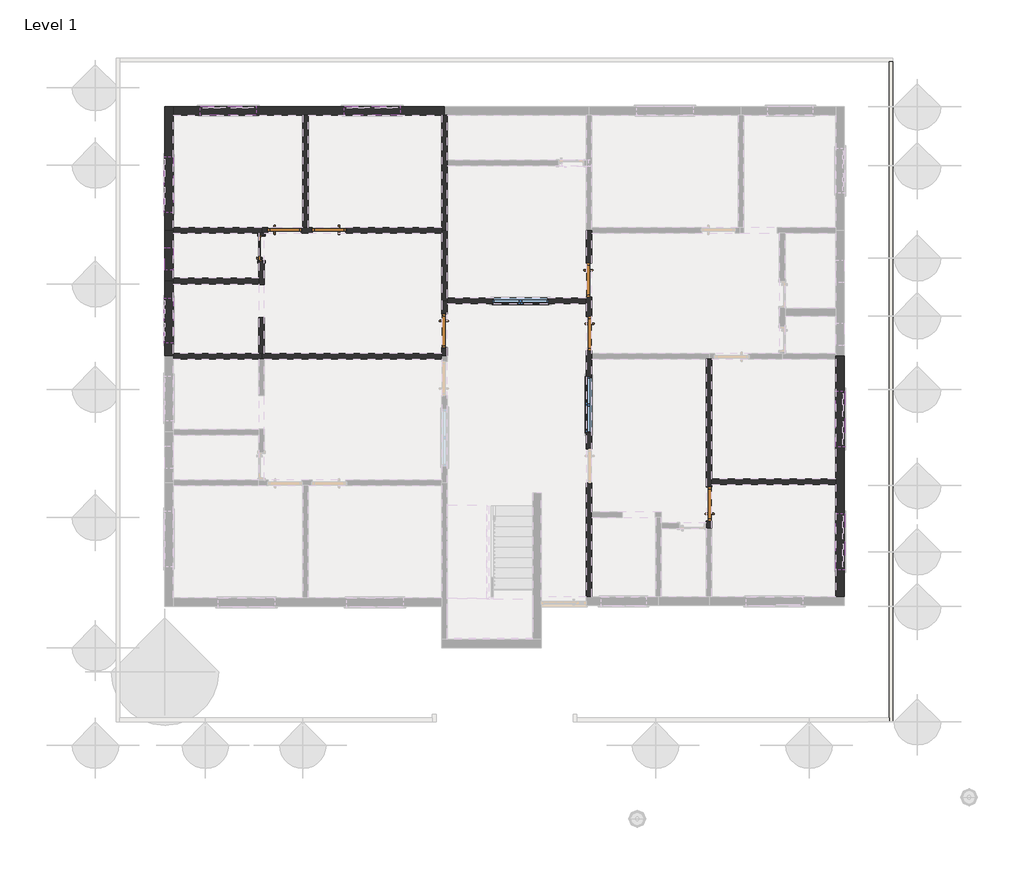
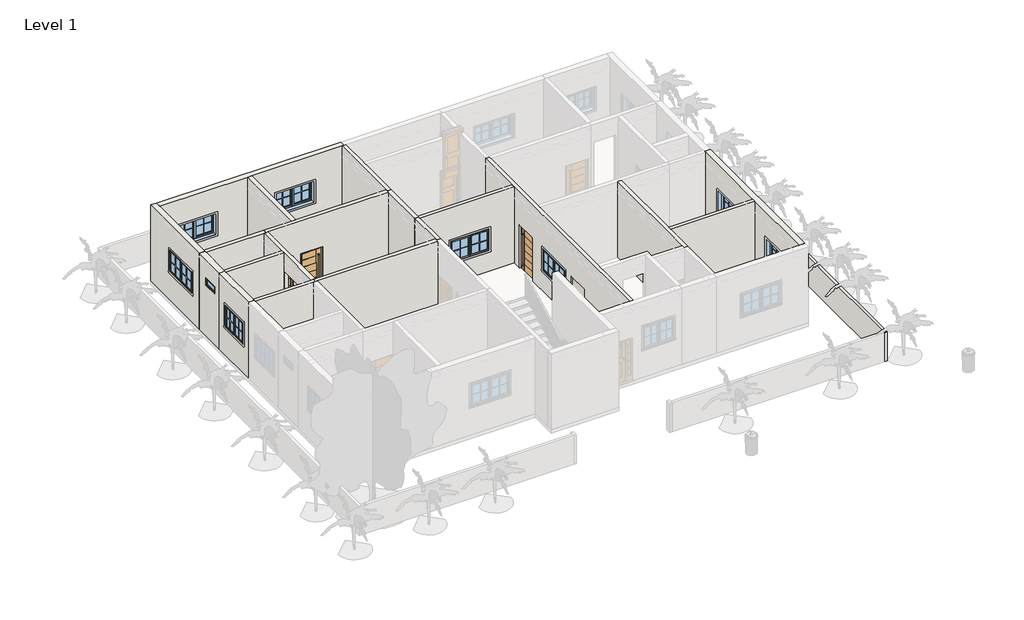
# One storey, part 2 of 5: 20 walls, 9 windows, 7 doors.
"""IFC4 building model written with IfcOpenShell, lengths in millimetres."""

from ifc_helpers import new_model, si_unit, origin, origin_with_axes, place, context, project, spatial, polyline, outline, extrude, faceted_brep, transform, mapped, element, save
from components import door_3_ad1505b7, door_3_44036f4b, door_57d9c04c, fixed_2_d9cafb20, m_window_awning_double_horizontal_4_0c6a2509, m_window_awning_double_horizontal_5_7c720334, m_window_awning_double_horizontal_5_337400f2

model = new_model("IFC4")

# Units and contexts
model_context = context("Model", 3, world=origin())
ifc_project = project(units=[si_unit("LENGTHUNIT", "METRE", prefix="MILLI")], contexts=[model_context])

# Site, building, storey
site = spatial("IfcSite", under=ifc_project)
building = spatial("IfcBuilding", under=site)
storey = spatial("IfcBuildingStorey", under=building, Name="Level 1", Elevation=0.0)

# Doors
placement = place(None, origin())
door_3_shape = door_3_ad1505b7(model_context)
element("IfcDoor", 1, ObjectType="3'", at=placement, inside=storey, context=model_context, shape_type="MappedRepresentation", body=[
    mapped(door_3_shape, transform((-21766.1847893, 19978.1922903, 0.0), x_axis=(1.0, 0.0, 0.0), y_axis=(0.0, 1.0, 0.0), z_axis=(0.0, 0.0, 1.0))),
])
element("IfcDoor", 2, ObjectType="3'", at=placement, inside=storey, context=model_context, shape_type="MappedRepresentation", body=[
    mapped(door_3_shape, transform((-13523.8847893, 17184.1922903, 0.0), x_axis=(0.0, -1.0, 0.0), y_axis=(1.0, 0.0, 0.0), z_axis=(0.0, 0.0, 1.0))),
])
door_3_2_shape = door_3_44036f4b(model_context)
element("IfcDoor", 3, ObjectType="3'", at=placement, inside=storey, context=model_context, shape_type="MappedRepresentation", body=[
    mapped(door_3_2_shape, transform((-20559.6847893, 19978.1922903, 0.0), x_axis=(-1.0, 0.0, 0.0), y_axis=(0.0, -1.0, 0.0), z_axis=(0.0, 0.0, 1.0))),
])
element("IfcDoor", 4, ObjectType="3'", at=placement, inside=storey, context=model_context, shape_type="MappedRepresentation", body=[
    mapped(door_3_2_shape, transform((-17435.4847893, 17260.3922903, 0.0), x_axis=(0.0, -1.0, 0.0), y_axis=(1.0, 0.0, 0.0), z_axis=(0.0, 0.0, 1.0))),
])
element("IfcDoor", 5, ObjectType="3'", at=placement, inside=storey, context=model_context, shape_type="MappedRepresentation", body=[
    mapped(door_3_2_shape, transform((-13523.8847893, 18631.9922903, 0.0), x_axis=(0.0, -1.0, 0.0), y_axis=(1.0, 0.0, 0.0), z_axis=(0.0, 0.0, 1.0))),
])
element("IfcDoor", 6, ObjectType="3'", at=placement, inside=storey, context=model_context, shape_type="MappedRepresentation", body=[
    mapped(door_3_2_shape, transform((-10272.6847893, 12574.0922903, 0.0), x_axis=(0.0, 1.0, 0.0), y_axis=(-1.0, 0.0, 0.0), z_axis=(0.0, 0.0, 1.0))),
])
door_shape = door_57d9c04c(model_context)
element("IfcDoor", 7, ObjectType="M_Door-Interior-Single-2_Panel-Wood : 2'2\"", at=placement, inside=storey, context=model_context, shape_type="MappedRepresentation", body=[
    mapped(door_shape, transform((-22391.6597893, 19495.5922903, 0.0), x_axis=(0.0, 1.0, 0.0), y_axis=(-1.0, 0.0, 0.0), z_axis=(0.0, 0.0, 1.0))),
])

# Walls
element("IfcWall", 8, ObjectType="Generic - 4\"", at=placement, inside=storey, context=model_context, shape_type="Brep", body=[
    faceted_brep([(-5395.8847893, 24550.1922903, -152.4), (-5395.8847893, 6770.1922903, -152.4), (-5395.8847893, 6668.5922903, -152.4), (-5395.8847893, 6668.5922903, 1066.8), (-5395.8847893, 6770.1922903, 1066.8), (-5395.8847893, 24550.1922903, 1066.8), (-5294.2847893, 24550.1922903, -152.4), (-5294.2847893, 24550.1922903, 1066.8), (-5294.2847893, 6668.5922903, 1066.8), (-5294.2847893, 6668.5922903, -152.4)], [[[0, 1, 2, 3, 4, 5]], [[6, 7, 8, 9]], [[2, 1, 0, 6, 9]], [[5, 4, 3, 8, 7]], [[0, 5, 7, 6]], [[3, 2, 9, 8]]]),
])
element("IfcWall", 9, ObjectType="Generic - 6\"", at=placement, inside=storey, context=model_context, shape_type="Brep", body=[
    faceted_brep([(-17511.6847893, 23102.3922903, 0.0), (-17511.6847893, 20054.3922903, 0.0), (-17511.6847893, 19978.1922903, 0.0), (-17511.6847893, 19978.1922903, 3200.4), (-17511.6847893, 20054.3922903, 3200.4), (-17511.6847893, 23102.3922903, 3200.4), (-17359.2847893, 23102.3922903, 0.0), (-17359.2847893, 23102.3922903, 3200.4), (-17359.2847893, 21883.1922903, 3200.4), (-17359.2847893, 21730.7922903, 3200.4), (-17359.2847893, 19978.1922903, 3200.4), (-17359.2847893, 19978.1922903, 0.0), (-17359.2847893, 21730.7922903, 0.0), (-17359.2847893, 21883.1922903, 0.0), (-17435.4847893, 23102.3922903, 0.0), (-17435.4847893, 23102.3922903, 3200.4)], [[[0, 1, 2, 3, 4, 5]], [[6, 7, 8, 9, 10, 11, 12, 13]], [[2, 1, 0, 14, 6, 13, 12, 11]], [[3, 2, 11, 10]], [[5, 4, 3, 10, 9, 8, 7, 15]], [[0, 5, 15, 7, 6, 14]]]),
])
element("IfcWall", 10, ObjectType="Generic - 6\"", at=placement, inside=storey, context=model_context, shape_type="Brep", body=[
    faceted_brep([(-24776.0847893, 19901.9922903, 0.0), (-22464.6847893, 19901.9922903, 0.0), (-22388.4847893, 19901.9922903, 0.0), (-22388.4847893, 19901.9922903, 3200.4), (-22464.6847893, 19901.9922903, 3200.4), (-24776.0847893, 19901.9922903, 3200.4), (-24776.0847893, 20054.3922903, 0.0), (-24776.0847893, 20054.3922903, 3200.4), (-22388.4847893, 20054.3922903, 3200.4), (-22388.4847893, 20054.3922903, 0.0), (-24776.0847893, 19978.1922903, 0.0), (-24776.0847893, 19978.1922903, 3200.4)], [[[0, 1, 2, 3, 4, 5]], [[6, 7, 8, 9]], [[2, 1, 0, 10, 6, 9]], [[3, 2, 9, 8]], [[5, 4, 3, 8, 7, 11]], [[0, 5, 11, 7, 6, 10]]]),
])
element("IfcWall", 11, ObjectType="Generic - 6\"", at=placement, inside=storey, context=model_context, shape_type="SweptSolid", body=[
    extrude(outline(polyline([(-21270.8847893, 20054.3922903), (-21270.8847893, 23102.3922903), (-21118.4847893, 23102.3922903), (-21118.4847893, 20054.3922903), (-21270.8847893, 20054.3922903)])), origin_with_axes(), (0.0, 0.0, 1.0), 3200.4),
])
element("IfcWall", 12, ObjectType="Generic - 6\"", at=placement, inside=storey, context=model_context, shape_type="Brep", body=[
    faceted_brep([(-24776.0847893, 16498.3922903, 0.0), (-22464.6847893, 16498.3922903, 0.0), (-22388.4847893, 16498.3922903, 0.0), (-22388.4847893, 16498.3922903, 3200.4), (-22464.6847893, 16498.3922903, 3200.4), (-24776.0847893, 16498.3922903, 3200.4), (-24776.0847893, 16650.7922903, 0.0), (-24776.0847893, 16650.7922903, 3200.4), (-22464.6847893, 16650.7922903, 3200.4), (-22388.4847893, 16650.7922903, 3200.4), (-22388.4847893, 16650.7922903, 0.0), (-22464.6847893, 16650.7922903, 0.0), (-24776.0847893, 16574.5922903, 0.0), (-24776.0847893, 16574.5922903, 3200.4)], [[[0, 1, 2, 3, 4, 5]], [[6, 7, 8, 9, 10, 11]], [[2, 1, 0, 12, 6, 11, 10]], [[3, 2, 10, 9]], [[5, 4, 3, 9, 8, 7, 13]], [[0, 5, 13, 7, 6, 12]]]),
])
element("IfcWall", 13, ObjectType="Generic - 6\"", at=placement, inside=storey, context=model_context, shape_type="Brep", body=[
    faceted_brep([(-24776.0847893, 18530.3922903, 0.0), (-22464.6847893, 18530.3922903, 0.0), (-22464.6847893, 18530.3922903, 3200.4), (-24776.0847893, 18530.3922903, 3200.4), (-24776.0847893, 18682.7922903, 0.0), (-24776.0847893, 18682.7922903, 3200.4), (-22464.6847893, 18682.7922903, 3200.4), (-22464.6847893, 18682.7922903, 0.0), (-24776.0847893, 18606.5922903, 0.0), (-24776.0847893, 18606.5922903, 3200.4)], [[[0, 1, 2, 3]], [[4, 5, 6, 7]], [[1, 0, 8, 4, 7]], [[3, 2, 6, 5, 9]], [[0, 3, 9, 5, 4, 8]], [[2, 1, 7, 6]]]),
])
element("IfcWall", 14, ObjectType="Generic - 6\"", at=placement, inside=storey, context=model_context, shape_type="Brep", body=[
    faceted_brep([(-22312.2847893, 19901.9922903, 3200.4), (-22312.2847893, 16650.7922903, 3200.4), (-22312.2847893, 16650.7922903, 0.0), (-22312.2847893, 17622.2018411, 0.0), (-22312.2847893, 17622.2018411, 2438.4), (-22312.2847893, 18518.7795946, 2438.4), (-22312.2847893, 18518.7795946, 0.0), (-22312.2847893, 19140.3922903, 0.0), (-22312.2847893, 19140.3922903, 1853.8), (-22312.2847893, 19850.7922903, 1853.8), (-22312.2847893, 19850.7922903, 0.0), (-22312.2847893, 19901.9922903, 0.0), (-22464.6847893, 16650.7922903, 3200.4), (-22464.6847893, 18530.3922903, 3200.4), (-22464.6847893, 18682.7922903, 3200.4), (-22464.6847893, 19901.9922903, 3200.4), (-22464.6847893, 19901.9922903, 0.0), (-22464.6847893, 19850.7922903, 0.0), (-22464.6847893, 19850.7922903, 1853.8), (-22464.6847893, 19140.3922903, 1853.8), (-22464.6847893, 19140.3922903, 0.0), (-22464.6847893, 18682.7922903, 0.0), (-22464.6847893, 18530.3922903, 0.0), (-22464.6847893, 18518.7795946, 0.0), (-22464.6847893, 18518.7795946, 2438.4), (-22464.6847893, 17622.2018411, 2438.4), (-22464.6847893, 17622.2018411, 0.0), (-22464.6847893, 16650.7922903, 0.0), (-22388.4847893, 16650.7922903, 0.0), (-22388.4847893, 19901.9922903, 0.0), (-22388.4847893, 19901.9922903, 3200.4), (-22388.4847893, 16650.7922903, 3200.4)], [[[0, 1, 2, 3, 4, 5, 6, 7, 8, 9, 10, 11]], [[12, 13, 14, 15, 16, 17, 18, 19, 20, 21, 22, 23, 24, 25, 26, 27]], [[2, 28, 27, 26, 3]], [[6, 23, 22, 21, 20, 7]], [[16, 29, 11, 10, 17]], [[1, 0, 30, 15, 14, 13, 12, 31]], [[0, 11, 29, 16, 15, 30]], [[2, 1, 31, 12, 27, 28]], [[9, 18, 17, 10]], [[18, 9, 8, 19]], [[19, 8, 7, 20]], [[4, 25, 24, 5]], [[25, 4, 3, 26]], [[5, 24, 23, 6]]]),
])
element("IfcWall", 15, ObjectType="Generic - 6\"", at=placement, inside=storey, context=model_context, shape_type="Brep", body=[
    faceted_brep([(-17359.2847893, 17996.9922903, 0.0), (-13600.0847893, 17996.9922903, 0.0), (-13600.0847893, 17996.9922903, 3200.4), (-17359.2847893, 17996.9922903, 3200.4), (-16140.0847893, 17996.9922903, 1814.4), (-14616.0847893, 17996.9922903, 1814.4), (-14616.0847893, 17996.9922903, 900.0), (-16140.0847893, 17996.9922903, 900.0), (-17359.2847893, 18149.3922903, 0.0), (-17359.2847893, 18149.3922903, 3200.4), (-13600.0847893, 18149.3922903, 3200.4), (-13600.0847893, 18149.3922903, 0.0), (-16140.0847893, 18149.3922903, 1814.4), (-16140.0847893, 18149.3922903, 900.0), (-14616.0847893, 18149.3922903, 900.0), (-14616.0847893, 18149.3922903, 1814.4), (-17359.2847893, 18073.1922903, 0.0), (-17359.2847893, 18073.1922903, 3200.4)], [[[0, 1, 2, 3], [4, 5, 6, 7]], [[8, 9, 10, 11], [12, 13, 14, 15]], [[1, 0, 16, 8, 11]], [[3, 2, 10, 9, 17]], [[0, 3, 17, 9, 8, 16]], [[2, 1, 11, 10]], [[13, 12, 4, 7]], [[14, 13, 7, 6]], [[15, 14, 6, 5]], [[12, 15, 5, 4]]]),
])
element("IfcWall", 16, ObjectType="Generic - 6\"", at=placement, inside=storey, context=model_context, shape_type="Brep", body=[
    faceted_brep([(-10348.8847893, 11913.6922903, 0.0), (-10348.8847893, 11913.6922903, 3200.4), (-10348.8847893, 12053.3922903, 3200.4), (-10348.8847893, 16498.3922903, 3200.4), (-10348.8847893, 16498.3922903, 0.0), (-10348.8847893, 13031.2922903, 0.0), (-10348.8847893, 13031.2922903, 1828.8), (-10348.8847893, 12116.8922903, 1828.8), (-10348.8847893, 12116.8922903, 0.0), (-10348.8847893, 12053.3922903, 0.0), (-10196.4847893, 11913.6922903, 3200.4), (-10196.4847893, 11913.6922903, 0.0), (-10196.4847893, 12116.8922903, 0.0), (-10196.4847893, 12116.8922903, 1828.8), (-10196.4847893, 13031.2922903, 1828.8), (-10196.4847893, 13031.2922903, 0.0), (-10196.4847893, 13094.7922903, 0.0), (-10196.4847893, 13247.1922903, 0.0), (-10196.4847893, 16498.3922903, 0.0), (-10196.4847893, 16498.3922903, 3200.4), (-10196.4847893, 13247.1922903, 3200.4), (-10196.4847893, 13094.7922903, 3200.4), (-10272.6847893, 16498.3922903, 0.0), (-10216.4847893, 13031.2922903, 0.0), (-10216.4847893, 13046.2922903, 0.0), (-10293.4847893, 13046.2922903, 0.0), (-10293.4847893, 13031.2922903, 0.0), (-10293.4847893, 12116.8922903, 0.0), (-10293.4847893, 12101.8922903, 0.0), (-10216.4847893, 12101.8922903, 0.0), (-10216.4847893, 12116.8922903, 0.0), (-10272.6847893, 16498.3922903, 3200.4), (-10216.4847893, 12116.8922903, 1828.8), (-10216.4847893, 13031.2922903, 1828.8), (-10293.4847893, 13031.2922903, 1828.8), (-10293.4847893, 12116.8922903, 1828.8), (-10216.4847893, 12101.8922903, 1843.8), (-10293.4847893, 12101.8922903, 1843.8), (-10293.4847893, 13046.2922903, 1843.8), (-10216.4847893, 13046.2922903, 1843.8)], [[[0, 1, 2, 3, 4, 5, 6, 7, 8, 9]], [[10, 11, 12, 13, 14, 15, 16, 17, 18, 19, 20, 21]], [[4, 22, 18, 17, 16, 15, 23, 24, 25, 26, 5]], [[11, 0, 9, 8, 27, 28, 29, 30, 12]], [[1, 0, 11, 10]], [[3, 2, 1, 10, 21, 20, 19, 31]], [[4, 3, 31, 19, 18, 22]], [[13, 32, 33, 14]], [[6, 34, 35, 7]], [[14, 33, 23, 15]], [[34, 6, 5, 26]], [[32, 13, 12, 30]], [[7, 35, 27, 8]], [[36, 37, 38, 39]], [[39, 38, 25, 24]], [[35, 34, 26, 25, 38, 37, 28, 27]], [[37, 36, 29, 28]], [[33, 32, 30, 29, 36, 39, 24, 23]]]),
])
element("IfcWall", 17, ObjectType="Generic - 6\"", at=placement, inside=storey, context=model_context, shape_type="SweptSolid", body=[
    extrude(outline(polyline([(-6843.6847893, 13094.7922903), (-10196.4847893, 13094.7922903), (-10196.4847893, 13247.1922903), (-6843.6847893, 13247.1922903), (-6843.6847893, 13094.7922903)])), origin_with_axes(), (0.0, 0.0, 1.0), 3200.4),
])
element("IfcWall", 18, ObjectType="Generic - 6\"", at=placement, inside=storey, context=model_context, shape_type="Brep", body=[
    faceted_brep([(-13600.0847893, 10046.7922903, 3200.4), (-13600.0847893, 17996.9922903, 3200.4), (-13600.0847893, 18149.3922903, 3200.4), (-13600.0847893, 19978.1922903, 3200.4), (-13600.0847893, 19978.1922903, 0.0), (-13600.0847893, 19089.1922903, 0.0), (-13600.0847893, 19089.1922903, 1828.8), (-13600.0847893, 18174.7922903, 1828.8), (-13600.0847893, 18174.7922903, 0.0), (-13600.0847893, 18149.3922903, 0.0), (-13600.0847893, 17996.9922903, 0.0), (-13600.0847893, 17641.3922903, 0.0), (-13600.0847893, 17641.3922903, 1828.8), (-13600.0847893, 16726.9922903, 1828.8), (-13600.0847893, 16726.9922903, 0.0), (-13600.0847893, 14059.9922903, 0.0), (-13600.0847893, 14059.9922903, 1828.8), (-13600.0847893, 13145.5922903, 1828.8), (-13600.0847893, 13145.5922903, 0.0), (-13600.0847893, 10046.7922903, 0.0), (-13600.0847893, 10046.7922903, 1828.8), (-13600.0847893, 16015.7922903, 1814.4), (-13600.0847893, 14491.7922903, 1814.4), (-13600.0847893, 14491.7922903, 900.0), (-13600.0847893, 16015.7922903, 900.0), (-13447.6847893, 19978.1922903, 3200.4), (-13447.6847893, 19901.9922903, 3200.4), (-13447.6847893, 16650.7922903, 3200.4), (-13447.6847893, 16498.3922903, 3200.4), (-13447.6847893, 12358.1922903, 3200.4), (-13447.6847893, 12205.7922903, 3200.4), (-13447.6847893, 10046.7922903, 3200.4), (-13447.6847893, 10046.7922903, 0.0), (-13447.6847893, 12205.7922903, 0.0), (-13447.6847893, 12358.1922903, 0.0), (-13447.6847893, 13145.5922903, 0.0), (-13447.6847893, 13145.5922903, 1828.8), (-13447.6847893, 14059.9922903, 1828.8), (-13447.6847893, 14059.9922903, 0.0), (-13447.6847893, 16498.3922903, 0.0), (-13447.6847893, 16650.7922903, 0.0), (-13447.6847893, 16726.9922903, 0.0), (-13447.6847893, 16726.9922903, 1828.8), (-13447.6847893, 17641.3922903, 1828.8), (-13447.6847893, 17641.3922903, 0.0), (-13447.6847893, 18174.7922903, 0.0), (-13447.6847893, 18174.7922903, 1828.8), (-13447.6847893, 19089.1922903, 1828.8), (-13447.6847893, 19089.1922903, 0.0), (-13447.6847893, 19901.9922903, 0.0), (-13447.6847893, 19978.1922903, 0.0), (-13447.6847893, 16015.7922903, 1814.4), (-13447.6847893, 16015.7922903, 900.0), (-13447.6847893, 14491.7922903, 900.0), (-13447.6847893, 14491.7922903, 1814.4), (-13544.6847893, 13145.5922903, 0.0), (-13544.6847893, 13130.5922903, 0.0), (-13467.6847893, 13130.5922903, 0.0), (-13467.6847893, 13145.5922903, 0.0), (-13544.6847893, 14059.9922903, 0.0), (-13544.6847893, 16726.9922903, 0.0), (-13544.6847893, 16711.9922903, 0.0), (-13467.6847893, 16711.9922903, 0.0), (-13467.6847893, 16726.9922903, 0.0), (-13467.6847893, 14059.9922903, 0.0), (-13467.6847893, 14074.9922903, 0.0), (-13544.6847893, 14074.9922903, 0.0), (-13544.6847893, 17641.3922903, 0.0), (-13580.0847893, 18174.7922903, 0.0), (-13580.0847893, 18159.7922903, 0.0), (-13503.0847893, 18159.7922903, 0.0), (-13503.0847893, 18174.7922903, 0.0), (-13467.6847893, 17641.3922903, 0.0), (-13467.6847893, 17656.3922903, 0.0), (-13544.6847893, 17656.3922903, 0.0), (-13503.0847893, 19089.1922903, 0.0), (-13503.0847893, 19104.1922903, 0.0), (-13580.0847893, 19104.1922903, 0.0), (-13580.0847893, 19089.1922903, 0.0), (-13544.6847893, 14059.9922903, 1828.8), (-13544.6847893, 13145.5922903, 1828.8), (-13467.6847893, 14059.9922903, 1828.8), (-13467.6847893, 13145.5922903, 1828.8), (-13467.6847893, 14074.9922903, 1843.8), (-13467.6847893, 13130.5922903, 1843.8), (-13544.6847893, 13130.5922903, 1843.8), (-13544.6847893, 14074.9922903, 1843.8), (-13544.6847893, 17641.3922903, 1828.8), (-13544.6847893, 16726.9922903, 1828.8), (-13467.6847893, 17641.3922903, 1828.8), (-13467.6847893, 16726.9922903, 1828.8), (-13467.6847893, 17656.3922903, 1843.8), (-13467.6847893, 16711.9922903, 1843.8), (-13544.6847893, 16711.9922903, 1843.8), (-13544.6847893, 17656.3922903, 1843.8), (-13580.0847893, 19089.1922903, 1828.8), (-13580.0847893, 18174.7922903, 1828.8), (-13503.0847893, 18174.7922903, 1828.8), (-13503.0847893, 19089.1922903, 1828.8), (-13580.0847893, 19104.1922903, 1843.8), (-13503.0847893, 19104.1922903, 1843.8), (-13503.0847893, 18159.7922903, 1843.8), (-13580.0847893, 18159.7922903, 1843.8)], [[[0, 1, 2, 3, 4, 5, 6, 7, 8, 9, 10, 11, 12, 13, 14, 15, 16, 17, 18, 19, 20], [21, 22, 23, 24]], [[25, 26, 27, 28, 29, 30, 31, 32, 33, 34, 35, 36, 37, 38, 39, 40, 41, 42, 43, 44, 45, 46, 47, 48, 49, 50], [51, 52, 53, 54]], [[32, 19, 18, 55, 56, 57, 58, 35, 34, 33]], [[59, 15, 14, 60, 61, 62, 63, 41, 40, 39, 38, 64, 65, 66]], [[67, 11, 10, 9, 8, 68, 69, 70, 71, 45, 44, 72, 73, 74]], [[4, 50, 49, 48, 75, 76, 77, 78, 5]], [[3, 2, 1, 0, 31, 30, 29, 28, 27, 26, 25]], [[4, 3, 25, 50]], [[0, 20, 19, 32, 31]], [[16, 79, 80, 17]], [[81, 37, 36, 82]], [[17, 80, 55, 18]], [[82, 36, 35, 58]], [[79, 16, 15, 59]], [[37, 81, 64, 38]], [[83, 84, 85, 86]], [[85, 84, 57, 56]], [[86, 85, 56, 55, 80, 79, 59, 66]], [[83, 86, 66, 65]], [[84, 83, 65, 64, 81, 82, 58, 57]], [[12, 87, 88, 13]], [[89, 43, 42, 90]], [[13, 88, 60, 14]], [[90, 42, 41, 63]], [[87, 12, 11, 67]], [[43, 89, 72, 44]], [[91, 92, 93, 94]], [[93, 92, 62, 61]], [[94, 93, 61, 60, 88, 87, 67, 74]], [[91, 94, 74, 73]], [[92, 91, 73, 72, 89, 90, 63, 62]], [[6, 95, 96, 7]], [[46, 97, 98, 47]], [[97, 46, 45, 71]], [[7, 96, 68, 8]], [[47, 98, 75, 48]], [[95, 6, 5, 78]], [[99, 100, 101, 102]], [[102, 101, 70, 69]], [[98, 97, 71, 70, 101, 100, 76, 75]], [[100, 99, 77, 76]], [[96, 95, 78, 77, 99, 102, 69, 68]], [[51, 54, 22, 21]], [[54, 53, 23, 22]], [[53, 52, 24, 23]], [[52, 51, 21, 24]]]),
])
element("IfcWall", 19, ObjectType="Generic - 6\"", at=placement, inside=storey, context=model_context, shape_type="Brep", body=[
    faceted_brep([(-22388.4847893, 16498.3922903, 0.0), (-22312.2847893, 16498.3922903, 0.0), (-17511.6847893, 16498.3922903, 0.0), (-17511.6847893, 16498.3922903, 3200.4), (-22312.2847893, 16498.3922903, 3200.4), (-22388.4847893, 16498.3922903, 3200.4), (-22388.4847893, 16650.7922903, 0.0), (-22388.4847893, 16650.7922903, 3200.4), (-22312.2847893, 16650.7922903, 3200.4), (-17511.6847893, 16650.7922903, 3200.4), (-17511.6847893, 16650.7922903, 0.0), (-22312.2847893, 16650.7922903, 0.0), (-17511.6847893, 16574.5922903, 0.0), (-17511.6847893, 16574.5922903, 3200.4)], [[[0, 1, 2, 3, 4, 5]], [[6, 7, 8, 9, 10, 11]], [[2, 1, 0, 6, 11, 10, 12]], [[5, 4, 3, 13, 9, 8, 7]], [[0, 5, 7, 6]], [[3, 2, 12, 10, 9, 13]]]),
])
element("IfcWall", 20, ObjectType="Generic - 6\"", at=placement, inside=storey, context=model_context, shape_type="Brep", body=[
    faceted_brep([(-17511.6847893, 19978.1922903, 0.0), (-17511.6847893, 19901.9922903, 0.0), (-17511.6847893, 18073.1922903, 0.0), (-17511.6847893, 18073.1922903, 3200.4), (-17511.6847893, 19901.9922903, 3200.4), (-17511.6847893, 19978.1922903, 3200.4), (-17359.2847893, 19978.1922903, 0.0), (-17359.2847893, 19978.1922903, 3200.4), (-17359.2847893, 18149.3922903, 3200.4), (-17359.2847893, 18073.1922903, 3200.4), (-17359.2847893, 18073.1922903, 0.0), (-17359.2847893, 18149.3922903, 0.0)], [[[0, 1, 2, 3, 4, 5]], [[6, 7, 8, 9, 10, 11]], [[2, 1, 0, 6, 11, 10]], [[3, 2, 10, 9]], [[5, 4, 3, 9, 8, 7]], [[0, 5, 7, 6]]]),
])
element("IfcWall", 21, ObjectType="Generic - 6\"", at=placement, inside=storey, context=model_context, shape_type="Brep", body=[
    faceted_brep([(-17511.6847893, 19901.9922903, 3200.4), (-22312.2847893, 19901.9922903, 3200.4), (-22388.4847893, 19901.9922903, 3200.4), (-22388.4847893, 19901.9922903, 0.0), (-22312.2847893, 19901.9922903, 0.0), (-22223.3847893, 19901.9922903, 0.0), (-22223.3847893, 19901.9922903, 1828.8), (-21308.9847893, 19901.9922903, 1828.8), (-21308.9847893, 19901.9922903, 0.0), (-21016.8847893, 19901.9922903, 0.0), (-21016.8847893, 19901.9922903, 1828.8), (-20102.4847893, 19901.9922903, 1828.8), (-20102.4847893, 19901.9922903, 0.0), (-17511.6847893, 19901.9922903, 0.0), (-22388.4847893, 20054.3922903, 3200.4), (-21270.8847893, 20054.3922903, 3200.4), (-21118.4847893, 20054.3922903, 3200.4), (-17511.6847893, 20054.3922903, 3200.4), (-17511.6847893, 20054.3922903, 0.0), (-20102.4847893, 20054.3922903, 0.0), (-20102.4847893, 20054.3922903, 1828.8), (-21016.8847893, 20054.3922903, 1828.8), (-21016.8847893, 20054.3922903, 0.0), (-21118.4847893, 20054.3922903, 0.0), (-21270.8847893, 20054.3922903, 0.0), (-21308.9847893, 20054.3922903, 0.0), (-21308.9847893, 20054.3922903, 1828.8), (-22223.3847893, 20054.3922903, 1828.8), (-22223.3847893, 20054.3922903, 0.0), (-22388.4847893, 20054.3922903, 0.0), (-17511.6847893, 19978.1922903, 0.0), (-20102.4847893, 19957.3922903, 0.0), (-20087.4847893, 19957.3922903, 0.0), (-20087.4847893, 20034.3922903, 0.0), (-20102.4847893, 20034.3922903, 0.0), (-21308.9847893, 19957.3922903, 0.0), (-21293.9847893, 19957.3922903, 0.0), (-21293.9847893, 20034.3922903, 0.0), (-21308.9847893, 20034.3922903, 0.0), (-21016.8847893, 20034.3922903, 0.0), (-21031.8847893, 20034.3922903, 0.0), (-21031.8847893, 19957.3922903, 0.0), (-21016.8847893, 19957.3922903, 0.0), (-22223.3847893, 20034.3922903, 0.0), (-22238.3847893, 20034.3922903, 0.0), (-22238.3847893, 19957.3922903, 0.0), (-22223.3847893, 19957.3922903, 0.0), (-17511.6847893, 19978.1922903, 3200.4), (-22223.3847893, 19957.3922903, 1828.8), (-21308.9847893, 19957.3922903, 1828.8), (-22223.3847893, 20034.3922903, 1828.8), (-21308.9847893, 20034.3922903, 1828.8), (-22238.3847893, 20034.3922903, 1843.8), (-21293.9847893, 20034.3922903, 1843.8), (-21293.9847893, 19957.3922903, 1843.8), (-22238.3847893, 19957.3922903, 1843.8), (-20102.4847893, 20034.3922903, 1828.8), (-21016.8847893, 20034.3922903, 1828.8), (-21016.8847893, 19957.3922903, 1828.8), (-20102.4847893, 19957.3922903, 1828.8), (-20087.4847893, 20034.3922903, 1843.8), (-20087.4847893, 19957.3922903, 1843.8), (-21031.8847893, 19957.3922903, 1843.8), (-21031.8847893, 20034.3922903, 1843.8)], [[[0, 1, 2, 3, 4, 5, 6, 7, 8, 9, 10, 11, 12, 13]], [[14, 15, 16, 17, 18, 19, 20, 21, 22, 23, 24, 25, 26, 27, 28, 29]], [[18, 30, 13, 12, 31, 32, 33, 34, 19]], [[8, 35, 36, 37, 38, 25, 24, 23, 22, 39, 40, 41, 42, 9]], [[3, 29, 28, 43, 44, 45, 46, 5, 4]], [[2, 1, 0, 47, 17, 16, 15, 14]], [[3, 2, 14, 29]], [[0, 13, 30, 18, 17, 47]], [[6, 48, 49, 7]], [[50, 27, 26, 51]], [[7, 49, 35, 8]], [[51, 26, 25, 38]], [[48, 6, 5, 46]], [[27, 50, 43, 28]], [[52, 53, 54, 55]], [[54, 53, 37, 36]], [[55, 54, 36, 35, 49, 48, 46, 45]], [[52, 55, 45, 44]], [[53, 52, 44, 43, 50, 51, 38, 37]], [[20, 56, 57, 21]], [[10, 58, 59, 11]], [[58, 10, 9, 42]], [[21, 57, 39, 22]], [[11, 59, 31, 12]], [[56, 20, 19, 34]], [[60, 61, 62, 63]], [[63, 62, 41, 40]], [[59, 58, 42, 41, 62, 61, 32, 31]], [[61, 60, 33, 32]], [[57, 56, 34, 33, 60, 63, 40, 39]]]),
])
element("IfcWall", 22, ObjectType="Generic - 6\"", at=placement, inside=storey, context=model_context, shape_type="Brep", body=[
    faceted_brep([(-17511.6847893, 16574.5922903, 0.0), (-17511.6847893, 16574.5922903, 3200.4), (-17511.6847893, 16650.7922903, 3200.4), (-17511.6847893, 18073.1922903, 3200.4), (-17511.6847893, 18073.1922903, 0.0), (-17511.6847893, 17717.5922903, 0.0), (-17511.6847893, 17717.5922903, 1828.8), (-17511.6847893, 16803.1922903, 1828.8), (-17511.6847893, 16803.1922903, 0.0), (-17511.6847893, 16650.7922903, 0.0), (-17359.2847893, 16574.5922903, 3200.4), (-17359.2847893, 16574.5922903, 0.0), (-17359.2847893, 16803.1922903, 0.0), (-17359.2847893, 16803.1922903, 1828.8), (-17359.2847893, 17717.5922903, 1828.8), (-17359.2847893, 17717.5922903, 0.0), (-17359.2847893, 17996.9922903, 0.0), (-17359.2847893, 18073.1922903, 0.0), (-17359.2847893, 18073.1922903, 3200.4), (-17359.2847893, 17996.9922903, 3200.4), (-17414.6847893, 17717.5922903, 0.0), (-17414.6847893, 17732.5922903, 0.0), (-17491.6847893, 17732.5922903, 0.0), (-17491.6847893, 17717.5922903, 0.0), (-17491.6847893, 16803.1922903, 0.0), (-17491.6847893, 16788.1922903, 0.0), (-17414.6847893, 16788.1922903, 0.0), (-17414.6847893, 16803.1922903, 0.0), (-17491.6847893, 17717.5922903, 1828.8), (-17491.6847893, 16803.1922903, 1828.8), (-17414.6847893, 16803.1922903, 1828.8), (-17414.6847893, 17717.5922903, 1828.8), (-17491.6847893, 17732.5922903, 1843.8), (-17414.6847893, 17732.5922903, 1843.8), (-17414.6847893, 16788.1922903, 1843.8), (-17491.6847893, 16788.1922903, 1843.8)], [[[0, 1, 2, 3, 4, 5, 6, 7, 8, 9]], [[10, 11, 12, 13, 14, 15, 16, 17, 18, 19]], [[4, 17, 16, 15, 20, 21, 22, 23, 5]], [[11, 0, 9, 8, 24, 25, 26, 27, 12]], [[1, 0, 11, 10]], [[3, 2, 1, 10, 19, 18]], [[4, 3, 18, 17]], [[6, 28, 29, 7]], [[13, 30, 31, 14]], [[30, 13, 12, 27]], [[7, 29, 24, 8]], [[14, 31, 20, 15]], [[28, 6, 5, 23]], [[32, 33, 34, 35]], [[35, 34, 26, 25]], [[31, 30, 27, 26, 34, 33, 21, 20]], [[33, 32, 22, 21]], [[29, 28, 23, 22, 32, 35, 25, 24]]]),
])
element("IfcWall", 23, ObjectType="Generic - 9\"", at=placement, inside=storey, context=model_context, shape_type="Brep", body=[
    faceted_brep([(-25004.6847893, 23330.9922903, 0.0), (-25004.6847893, 19978.1922903, 0.0), (-25004.6847893, 19978.1922903, 3200.4), (-25004.6847893, 23330.9922903, 3200.4), (-25004.6847893, 21984.7922903, 2133.5570313), (-25004.6847893, 20460.7922903, 2133.5570313), (-25004.6847893, 20460.7922903, 1219.1570313), (-25004.6847893, 21984.7922903, 1219.1570313), (-24776.0847893, 23330.9922903, 0.0), (-24776.0847893, 23330.9922903, 3200.4), (-24776.0847893, 23102.3922903, 3200.4), (-24776.0847893, 20054.3922903, 3200.4), (-24776.0847893, 19978.1922903, 3200.4), (-24776.0847893, 19978.1922903, 0.0), (-24776.0847893, 20054.3922903, 0.0), (-24776.0847893, 23102.3922903, 0.0), (-24776.0847893, 21984.7922903, 2133.5570313), (-24776.0847893, 21984.7922903, 1219.1570313), (-24776.0847893, 20460.7922903, 1219.1570313), (-24776.0847893, 20460.7922903, 2133.5570313)], [[[0, 1, 2, 3], [4, 5, 6, 7]], [[8, 9, 10, 11, 12, 13, 14, 15], [16, 17, 18, 19]], [[1, 0, 8, 15, 14, 13]], [[2, 1, 13, 12]], [[3, 2, 12, 11, 10, 9]], [[0, 3, 9, 8]], [[17, 16, 4, 7]], [[18, 17, 7, 6]], [[19, 18, 6, 5]], [[16, 19, 5, 4]]]),
])
element("IfcWall", 24, ObjectType="Generic - 9\"", at=placement, inside=storey, context=model_context, shape_type="Brep", body=[
    faceted_brep([(-6615.0847893, 10046.7922903, 0.0), (-6615.0847893, 16574.5922903, 0.0), (-6615.0847893, 16574.5922903, 3200.4), (-6615.0847893, 10046.7922903, 3200.4), (-6615.0847893, 10789.7422903, 2133.5570313), (-6615.0847893, 12313.7422903, 2133.5570313), (-6615.0847893, 12313.7422903, 1219.1570313), (-6615.0847893, 10789.7422903, 1219.1570313), (-6615.0847893, 14110.7922903, 2133.5570313), (-6615.0847893, 15634.7922903, 2133.5570313), (-6615.0847893, 15634.7922903, 1219.1570313), (-6615.0847893, 14110.7922903, 1219.1570313), (-6843.6847893, 10046.7922903, 0.0), (-6843.6847893, 10046.7922903, 3200.4), (-6843.6847893, 13094.7922903, 3200.4), (-6843.6847893, 13247.1922903, 3200.4), (-6843.6847893, 16498.3922903, 3200.4), (-6843.6847893, 16574.5922903, 3200.4), (-6843.6847893, 16574.5922903, 0.0), (-6843.6847893, 16498.3922903, 0.0), (-6843.6847893, 13247.1922903, 0.0), (-6843.6847893, 13094.7922903, 0.0), (-6843.6847893, 10789.7422903, 2133.5570313), (-6843.6847893, 10789.7422903, 1219.1570313), (-6843.6847893, 12313.7422903, 1219.1570313), (-6843.6847893, 12313.7422903, 2133.5570313), (-6843.6847893, 14110.7922903, 2133.5570313), (-6843.6847893, 14110.7922903, 1219.1570313), (-6843.6847893, 15634.7922903, 1219.1570313), (-6843.6847893, 15634.7922903, 2133.5570313)], [[[0, 1, 2, 3], [4, 5, 6, 7], [8, 9, 10, 11]], [[12, 13, 14, 15, 16, 17, 18, 19, 20, 21], [22, 23, 24, 25], [26, 27, 28, 29]], [[1, 0, 12, 21, 20, 19, 18]], [[2, 1, 18, 17]], [[3, 2, 17, 16, 15, 14, 13]], [[0, 3, 13, 12]], [[23, 22, 4, 7]], [[24, 23, 7, 6]], [[25, 24, 6, 5]], [[22, 25, 5, 4]], [[27, 26, 8, 11]], [[28, 27, 11, 10]], [[29, 28, 10, 9]], [[26, 29, 9, 8]]]),
])
element("IfcWall", 25, ObjectType="Generic - 9\"", at=placement, inside=storey, context=model_context, shape_type="Brep", body=[
    faceted_brep([(-17435.4847893, 23330.9922903, 0.0), (-24776.0847893, 23330.9922903, 0.0), (-24776.0847893, 23330.9922903, 3200.4), (-17435.4847893, 23330.9922903, 3200.4), (-22528.1847893, 23330.9922903, 2133.5570313), (-24052.1847893, 23330.9922903, 2133.5570313), (-24052.1847893, 23330.9922903, 1219.1570313), (-22528.1847893, 23330.9922903, 1219.1570313), (-18629.2847893, 23330.9922903, 2133.5570313), (-20153.2847893, 23330.9922903, 2133.5570313), (-20153.2847893, 23330.9922903, 1219.1570313), (-18629.2847893, 23330.9922903, 1219.1570313), (-17435.4847893, 23102.3922903, 0.0), (-17435.4847893, 23102.3922903, 3200.4), (-17511.6847893, 23102.3922903, 3200.4), (-21118.4847893, 23102.3922903, 3200.4), (-21270.8847893, 23102.3922903, 3200.4), (-24776.0847893, 23102.3922903, 3200.4), (-24776.0847893, 23102.3922903, 0.0), (-21270.8847893, 23102.3922903, 0.0), (-21118.4847893, 23102.3922903, 0.0), (-17511.6847893, 23102.3922903, 0.0), (-22528.1847893, 23102.3922903, 2133.5570313), (-22528.1847893, 23102.3922903, 1219.1570313), (-24052.1847893, 23102.3922903, 1219.1570313), (-24052.1847893, 23102.3922903, 2133.5570313), (-18629.2847893, 23102.3922903, 2133.5570313), (-18629.2847893, 23102.3922903, 1219.1570313), (-20153.2847893, 23102.3922903, 1219.1570313), (-20153.2847893, 23102.3922903, 2133.5570313)], [[[0, 1, 2, 3], [4, 5, 6, 7], [8, 9, 10, 11]], [[12, 13, 14, 15, 16, 17, 18, 19, 20, 21], [22, 23, 24, 25], [26, 27, 28, 29]], [[1, 0, 12, 21, 20, 19, 18]], [[3, 2, 17, 16, 15, 14, 13]], [[0, 3, 13, 12]], [[2, 1, 18, 17]], [[22, 25, 5, 4]], [[25, 24, 6, 5]], [[24, 23, 7, 6]], [[23, 22, 4, 7]], [[26, 29, 9, 8]], [[29, 28, 10, 9]], [[28, 27, 11, 10]], [[27, 26, 8, 11]]]),
])
element("IfcWall", 26, ObjectType="Generic - 9\"", at=placement, inside=storey, context=model_context, shape_type="Brep", body=[
    faceted_brep([(-25004.6847893, 18606.5922903, 0.0), (-25004.6847893, 16574.5922903, 0.0), (-25004.6847893, 16574.5922903, 3200.4), (-25004.6847893, 18606.5922903, 3200.4), (-25004.6847893, 18149.3922903, 2133.6), (-25004.6847893, 16930.1922903, 2133.6), (-25004.6847893, 16930.1922903, 1219.2), (-25004.6847893, 18149.3922903, 1219.2), (-24776.0847893, 18606.5922903, 0.0), (-24776.0847893, 18606.5922903, 3200.4), (-24776.0847893, 18530.3922903, 3200.4), (-24776.0847893, 16650.7922903, 3200.4), (-24776.0847893, 16574.5922903, 3200.4), (-24776.0847893, 16574.5922903, 0.0), (-24776.0847893, 16650.7922903, 0.0), (-24776.0847893, 18530.3922903, 0.0), (-24776.0847893, 18149.3922903, 2133.6), (-24776.0847893, 18149.3922903, 1219.2), (-24776.0847893, 16930.1922903, 1219.2), (-24776.0847893, 16930.1922903, 2133.6)], [[[0, 1, 2, 3], [4, 5, 6, 7]], [[8, 9, 10, 11, 12, 13, 14, 15], [16, 17, 18, 19]], [[1, 0, 8, 15, 14, 13]], [[2, 1, 13, 12]], [[3, 2, 12, 11, 10, 9]], [[0, 3, 9, 8]], [[16, 19, 5, 4]], [[19, 18, 6, 5]], [[18, 17, 7, 6]], [[17, 16, 4, 7]]]),
])
element("IfcWall", 27, ObjectType="Generic - 9\"", at=placement, inside=storey, context=model_context, shape_type="Brep", body=[
    faceted_brep([(-25004.6847893, 19978.1922903, 0.0), (-25004.6847893, 18606.5922903, 0.0), (-25004.6847893, 18606.5922903, 3200.4), (-25004.6847893, 19978.1922903, 3200.4), (-25004.6847893, 19520.9922903, 2438.4), (-25004.6847893, 18911.3922903, 2438.4), (-25004.6847893, 18911.3922903, 2133.6), (-25004.6847893, 19520.9922903, 2133.6), (-24776.0847893, 19978.1922903, 0.0), (-24776.0847893, 19978.1922903, 3200.4), (-24776.0847893, 19901.9922903, 3200.4), (-24776.0847893, 18682.7922903, 3200.4), (-24776.0847893, 18606.5922903, 3200.4), (-24776.0847893, 18606.5922903, 0.0), (-24776.0847893, 18682.7922903, 0.0), (-24776.0847893, 19901.9922903, 0.0), (-24776.0847893, 19520.9922903, 2438.4), (-24776.0847893, 19520.9922903, 2133.6), (-24776.0847893, 18911.3922903, 2133.6), (-24776.0847893, 18911.3922903, 2438.4)], [[[0, 1, 2, 3], [4, 5, 6, 7]], [[8, 9, 10, 11, 12, 13, 14, 15], [16, 17, 18, 19]], [[1, 0, 8, 15, 14, 13]], [[2, 1, 13, 12]], [[3, 2, 12, 11, 10, 9]], [[0, 3, 9, 8]], [[16, 19, 5, 4]], [[19, 18, 6, 5]], [[18, 17, 7, 6]], [[17, 16, 4, 7]]]),
])

# Windows
fixed_2_shape = fixed_2_d9cafb20(model_context)
element("IfcWindow", 28, ObjectType="Fixed : 2'", at=placement, inside=storey, context=model_context, shape_type="MappedRepresentation", body=[
    mapped(fixed_2_shape, transform((-24890.3847893, 19254.2922903, 0.0), x_axis=(0.0, 1.0, 0.0), y_axis=(-1.0, 0.0, 0.0), z_axis=(0.0, 0.0, 1.0))),
])
m_window_awning_double_horizontal_4_shape = m_window_awning_double_horizontal_4_0c6a2509(model_context)
element("IfcWindow", 29, ObjectType="M_Window-Awning-Double-Horizontal : 4'", at=placement, inside=storey, context=model_context, shape_type="MappedRepresentation", body=[
    mapped(m_window_awning_double_horizontal_4_shape, transform((-24890.3847893, 17539.7922903, 319.2), x_axis=(0.0, 1.0, 0.0), y_axis=(-1.0, 0.0, 0.0), z_axis=(0.0, 0.0, 1.0))),
])
m_window_awning_double_horizontal_5_shape = m_window_awning_double_horizontal_5_7c720334(model_context)
element("IfcWindow", 30, ObjectType="M_Window-Awning-Double-Horizontal : 5'", at=placement, inside=storey, context=model_context, shape_type="MappedRepresentation", body=[
    mapped(m_window_awning_double_horizontal_5_shape, transform((-23290.1847893, 23216.6922903, 319.1570312), x_axis=(1.0, 0.0, 0.0), y_axis=(0.0, 1.0, 0.0), z_axis=(0.0, 0.0, 1.0))),
])
element("IfcWindow", 31, ObjectType="M_Window-Awning-Double-Horizontal : 5'", at=placement, inside=storey, context=model_context, shape_type="MappedRepresentation", body=[
    mapped(m_window_awning_double_horizontal_5_shape, transform((-24890.3847893, 21222.7922903, 319.1570312), x_axis=(0.0, 1.0, 0.0), y_axis=(-1.0, 0.0, 0.0), z_axis=(0.0, 0.0, 1.0))),
])
element("IfcWindow", 32, ObjectType="M_Window-Awning-Double-Horizontal : 5'", at=placement, inside=storey, context=model_context, shape_type="MappedRepresentation", body=[
    mapped(m_window_awning_double_horizontal_5_shape, transform((-6729.3847893, 11551.7422903, 319.1570312), x_axis=(0.0, -1.0, 0.0), y_axis=(1.0, 0.0, 0.0), z_axis=(0.0, 0.0, 1.0))),
])
element("IfcWindow", 33, ObjectType="M_Window-Awning-Double-Horizontal : 5'", at=placement, inside=storey, context=model_context, shape_type="MappedRepresentation", body=[
    mapped(m_window_awning_double_horizontal_5_shape, transform((-6729.3847893, 14872.7922903, 319.1570312), x_axis=(0.0, -1.0, 0.0), y_axis=(1.0, 0.0, 0.0), z_axis=(0.0, 0.0, 1.0))),
])
element("IfcWindow", 34, ObjectType="M_Window-Awning-Double-Horizontal : 5'", at=placement, inside=storey, context=model_context, shape_type="MappedRepresentation", body=[
    mapped(m_window_awning_double_horizontal_5_shape, transform((-19391.2847893, 23216.6922903, 319.1570312), x_axis=(1.0, 0.0, 0.0), y_axis=(0.0, 1.0, 0.0), z_axis=(0.0, 0.0, 1.0))),
])
m_window_awning_double_horizontal_5_2_shape = m_window_awning_double_horizontal_5_337400f2(model_context)
element("IfcWindow", 35, ObjectType="M_Window-Awning-Double-Horizontal : 5'", at=placement, inside=storey, context=model_context, shape_type="MappedRepresentation", body=[
    mapped(m_window_awning_double_horizontal_5_2_shape, transform((-15378.0847893, 18073.1922903, 0.0), x_axis=(-1.0, 0.0, 0.0), y_axis=(0.0, -1.0, 0.0), z_axis=(0.0, 0.0, 1.0))),
])
element("IfcWindow", 36, ObjectType="M_Window-Awning-Double-Horizontal : 5'", at=placement, inside=storey, context=model_context, shape_type="MappedRepresentation", body=[
    mapped(m_window_awning_double_horizontal_5_2_shape, transform((-13523.8847893, 15253.7922903, 0.0), x_axis=(0.0, 1.0, 0.0), y_axis=(-1.0, 0.0, 0.0), z_axis=(0.0, 0.0, 1.0))),
])

save(model, "model.ifc")

# Revit data of these elements
# Type "3'"
#   Type Mark = "9"
#   Water resistance = "up to Class E900, EN 12208:2001"
#   Uniclass2015Version = "v1.21"
#   Uniclass2015Reference = "Ss_25_30_20_30"
#   Uniclass2015Description = "Frame and door leaf system"
#   URL = "www.aluprof.com"
#   Type IFC Predefined Type = "USERDEFINED"
#   Right-hand / Left-hand door [instance default] = ""
#   Resistance to wind load = "up to Class C5/B5, EN 12210:2001"
#   Insert type = "ST"
#   Hardware [instance default] = ""
#   Product page = "https://aluprof.com/en/architects/offer/window-and-door-systems/panel-doors#visualisation"
#   Operation = "SinglePanelOutwardOpening"
#   Opening type = "Outward"
#   NBSReference = "25-50-20/125"
#   NBSDescription = "Frame and door leaf system"
#   Important = "The actual acceptable construction dimensions are dependent on the selection of profiles and hardware, glazing type, construction weight and the construction’s operating conditions. These should be determined by a suitably qualified person, and using ALUPROF’s calculation software"
#   IfcExportType = "USERDEFINED"
#   IfcExportAs = "IfcDoorType"
#   Handle type [instance default] = ""
#   Manufacturer = "ALUPROF SA"
#   Export Type to IFC As = "IfcDoorType"
#   Door sill type [instance default] = ""
#   Description = "External single-leaf panel door outward opening"
#   Model = "MB-86 ST Panel Door AD07"
#   Content of the recyclate in the material = "69.2%"
#   COBie.Type.WarrantyDurationParts = ""
#   COBie.Type.Name = ""
#   COBie.Type.Manufacturer = "ALUPROF SA"
#   COBie.Space.Name = ""
#   COBie.Floor.Name = ""
#   COBie.Facility.Name = ""
#   COBie.CreatedOn = ""
#   COBie.Component.WarrantyStartDate = ""
#   COBie.Component.Name = "MB-86 ST Panel Door AD07"
#   Burglar resistance = "RC2"
#   Air permeability = "up to Class 4, EN 12207:2001"
#   Width of the active leaf = 2' - 8.17717"
#   Placement in wall = 0' - 0.7874"
#   Thickness = 0' - 3.0315"
#   Height of the opening sash = 5' - 9.44094"
#   Handle Offset = 3' - 5.33858"
#   Rough Height = 6' - 2.40945"
#   Rough Width = 3' - 1.1811"
#   Height = 6' - 0"
#   Width = 3' - 0"
#   Construction depth = 0' - 3.0315"
#   Clear opening width = 2' - 3.94882"
#   Clear opening height = 5' - 8.47638"
#   Height of the array = 0' - 11.08136"
#   Schedule No. [instance default] = 1
#   Handrail [instance default] = yes
#   IsExternal = yes
#   Handle [instance default] = no
#   Door closer [instance default] = no
#   Function = 1
#   COBie.Type = yes
#   COBie = yes
#   Access control [instance default] = no
#   Panel = element 380783
#   Wall Closure = (empty or 0)
# Type "M_Door-Interior-Single-2_Panel-Wood : 2'2\""
#   Type Mark = "11"
#   Assembly Code = "C1020300"
#   Analytic Construction = "Wooden"
#   Top Rail = 0' - 4.72441"
#   Thickness = 0' - 1.37795"
#   Thermal Resistance (R) = 2.5876 (h·ft²·°F)/BTU
#   Swing Angle [instance default] = 90.00°
#   Stiles = 0' - 4.72441"
#   Rough Width = 2' - 3.9685"
#   Rough Height = 6' - 0.98425"
#   Lock Rail = 0' - 7.87402"
#   Height = 6' - 0"
#   Width = 2' - 2"
#   Heat Transfer Coefficient (U) = 0.3865 BTU/(h·ft²·°F)
#   Bottom Rail = 0' - 9.05512"
#   Trim Material = Cherry
#   Panel Material = Cherry
#   Frame Material = Cherry
#   Door Handle Material = Aluminum
#   Visual Light Transmittance = 0
#   Solar Heat Gain Coefficient = 0
#   Wall Closure = (empty or 0)
#   Function = (empty or 0)
# Type "Generic - 4\""
#   Assembly Code = "B2010"
#   Layers, outside or top first: 0' - 4" no material (function 1)
# Type "Generic - 6\""
#   Assembly Code = "B2010"
#   Layers, outside or top first: 0' - 6" no material (function 1)
# Type "Generic - 9\""
#   Assembly Code = "B2010"
#   Layers, outside or top first: 0' - 9" no material (function 1)
# Type "Fixed : 2'"
#   Type Mark = "22"
#   Construction Type Id = "GSP4R"
#   Assembly Code = "B2020100"
#   Analytic Construction = "1/8 in Pilkington single glazing"
#   Visual Light Transmittance = 0.9
#   Solar Heat Gain Coefficient = 0.78
#   Heat Transfer Coefficient (U) = 0.6496 BTU/(h·ft²·°F)
#   Height = 1' - 0"
#   Default Sill Height = 7' - 0"
#   Width = 2' - 0"
#   Window Inset = 0' - 0 3/4"
#   Define Thermal Properties by = 1
#   Glass Pane Material = Glass
#   Sash Material = Sash
#   Wall Closure = (empty or 0)
# Type "M_Window-Awning-Double-Horizontal : 4'"
#   Type Mark = "21"
#   Fire Rating = "0.5h"
#   Assembly Code = "B2020100"
#   Analytic Construction = "Double glazing - domestic"
#   Window Inset [instance default] = 0' - 0"
#   Wall Thickness [instance default] = 0' - 5.90551"
#   Interior Wall Closure [instance default] = 0' - 2.15551"
#   Half Width = 2' - 0"
#   Visual Light Transmittance = 0.81
#   Thermal Resistance (R) = 1.8146 (h·ft²·°F)/BTU
#   Solar Heat Gain Coefficient = 0.76
#   Rough Width = 4' - 0.59055"
#   Rough Height = 3' - 0.59055"
#   Height = 3' - 0"
#   Heat Transfer Coefficient (U) = 0.5511 BTU/(h·ft²·°F)
#   Frame Extension [instance default] = 0' - 0 1/4"
#   Exterior Wall Closure [instance default] = 0' - 1 1/4"
#   Extension Jamb [instance default] = 0' - 2.15551"
#   Default Sill Height = 2' - 11.43307"
#   Width = 4' - 0"
#   Muntin Visibility = yes
#   Interior Trim Visibility [instance default] = yes
#   Exterior Trim Visibility [instance default] = yes
#   Extension Jamb Visibility [instance default] = yes
#   Interior Trim Material = Wood - Stained
#   Muntin Pattern = M_Muntin Pattern_2x2 : M_Muntin Pattern_2x2
#   Interior Trim = M_Trim-Window-Interior-Flat : Picture Frame
#   Interior Frame Material = Wood - Stained
#   Glass Panel Material = Glass
#   Exterior Trim Material = Clad - White
#   Exterior Trim = M_Trim-Window-Exterior-Flat : with Sill
#   Exterior Frame Material = Clad - White
#   Wall Closure = (empty or 0)
# Type "M_Window-Awning-Double-Horizontal : 5'"
#   Type Mark = "19"
#   Fire Rating = "0.5h"
#   Assembly Code = "B2020100"
#   Analytic Construction = "Double glazing - domestic"
#   Window Inset [instance default] = 0' - 0"
#   Wall Thickness [instance default] = 0' - 5.90551"
#   Interior Wall Closure [instance default] = 0' - 2.15551"
#   Half Width = 2' - 6"
#   Visual Light Transmittance = 0.81
#   Thermal Resistance (R) = 1.8146 (h·ft²·°F)/BTU
#   Solar Heat Gain Coefficient = 0.76
#   Rough Width = 5' - 0.59055"
#   Rough Height = 3' - 0.59055"
#   Height = 3' - 0"
#   Heat Transfer Coefficient (U) = 0.5511 BTU/(h·ft²·°F)
#   Frame Extension [instance default] = 0' - 0 1/4"
#   Exterior Wall Closure [instance default] = 0' - 1 1/4"
#   Extension Jamb [instance default] = 0' - 2.15551"
#   Default Sill Height = 2' - 11.43307"
#   Width = 5' - 0"
#   Muntin Visibility = yes
#   Interior Trim Visibility [instance default] = yes
#   Exterior Trim Visibility [instance default] = yes
#   Extension Jamb Visibility [instance default] = yes
#   Interior Trim Material = Wood - Stained
#   Muntin Pattern = M_Muntin Pattern_2x2 : M_Muntin Pattern_2x2
#   Interior Trim = M_Trim-Window-Interior-Flat : Picture Frame
#   Interior Frame Material = Wood - Stained
#   Glass Panel Material = Glass
#   Exterior Trim Material = Clad - White
#   Exterior Trim = M_Trim-Window-Exterior-Flat : with Sill
#   Exterior Frame Material = Clad - White
#   Wall Closure = (empty or 0)
# Elements 1, 2, 3, 4, 5, 6 (IfcDoor, "3'")
#   Right-hand / Left-hand door = ""
#   Hardware = ""
#   Handle type = ""
#   Door sill type = ""
#   Schedule No. = 1
#   Handrail = yes
#   Handle = no
#   Door closer = no
#   Access control = no
#   Phase Created = New Construction
# Element 7 (IfcDoor, "M_Door-Interior-Single-2_Panel-Wood : 2'2\"")
#   Swing Angle = 90.00°
#   Phase Created = New Construction
#   Materials on its faces: "Cherry", "Aluminum"
# Element 8 (IfcWall, "Generic - 4\"")
#   built-in parameter 1001111 = -0' - 6"
#   Top Offset = 0' - 0"
#   Base Offset = -0' - 6"
#   Unconnected Height = 4' - 0"
#   wall height = 4' - 0"
#   Phase Created = New Construction
#   Base Constraint = Level 1
#   Materials on its faces: "Default Wall"
# Element 9 (IfcWall, "Generic - 6\"")
#   Top Offset = 0' - 0"
#   Base Offset = 0' - 0"
#   Unconnected Height = 10' - 6"
#   wall height = 10' - 6"
#   Phase Created = New Construction
#   Base Constraint = Level 1
#   Materials on its faces: "Default Wall", "BRW2"
# Element 10 (IfcWall, "Generic - 6\"")
#   Top Offset = 0' - 0"
#   Base Offset = 0' - 0"
#   Unconnected Height = 10' - 6"
#   wall height = 10' - 6"
#   Phase Created = New Construction
#   Base Constraint = Level 1
#   Materials on its faces: "Default Wall", "BW1", "BRW2"
# Elements 11, 15 (IfcWall, "Generic - 6\"")
#   Top Offset = 0' - 0"
#   Base Offset = 0' - 0"
#   Unconnected Height = 10' - 6"
#   wall height = 10' - 6"
#   Phase Created = New Construction
#   Base Constraint = Level 1
#   Materials on its faces: "Default Wall", "BRW1"
# Element 12 (IfcWall, "Generic - 6\"")
#   Top Offset = 0' - 0"
#   Base Offset = 0' - 0"
#   Unconnected Height = 10' - 6"
#   wall height = 10' - 6"
#   Phase Created = New Construction
#   Base Constraint = Level 1
#   Materials on its faces: "Default Wall", "KW2", "KW1"
# Element 13 (IfcWall, "Generic - 6\"")
#   Top Offset = 0' - 0"
#   Base Offset = 0' - 0"
#   Unconnected Height = 10' - 6"
#   wall height = 10' - 6"
#   Phase Created = New Construction
#   Base Constraint = Level 1
#   Materials on its faces: "Default Wall", "KW2", "BW1"
# Element 14 (IfcWall, "Generic - 6\"")
#   Top Offset = 0' - 0"
#   Base Offset = 0' - 0"
#   Unconnected Height = 10' - 6"
#   wall height = 10' - 6"
#   Phase Created = New Construction
#   Base Constraint = Level 1
#   Materials on its faces: "Default Wall", "LVW1", "KW1"
# Element 16 (IfcWall, "Generic - 6\"")
#   Top Offset = 0' - 0"
#   Base Offset = 0' - 0"
#   Unconnected Height = 10' - 6"
#   wall height = 10' - 6"
#   Phase Created = New Construction
#   Base Constraint = Level 1
#   Materials on its faces: "Default Wall", "LVW2", "BRW4"
# Element 17 (IfcWall, "Generic - 6\"")
#   Top Offset = 0' - 0"
#   Base Offset = 0' - 0"
#   Unconnected Height = 10' - 6"
#   wall height = 10' - 6"
#   Phase Created = New Construction
#   Base Constraint = Level 1
#   Materials on its faces: "Default Wall", "BRW3"
# Element 18 (IfcWall, "Generic - 6\"")
#   Top Offset = 0' - 0"
#   Base Offset = 0' - 0"
#   Unconnected Height = 10' - 6"
#   wall height = 10' - 6"
#   Phase Created = New Construction
#   Base Constraint = Level 1
#   Materials on its faces: "Default Wall", "BRW1", "LVW2", "OW1"
# Element 19 (IfcWall, "Generic - 6\"")
#   Top Offset = 0' - 0"
#   Base Offset = 0' - 0"
#   Unconnected Height = 10' - 6"
#   wall height = 10' - 6"
#   Phase Created = New Construction
#   Base Constraint = Level 1
#   Materials on its faces: "Default Wall", "LVW1"
# Elements 20, 21 (IfcWall, "Generic - 6\"")
#   Top Offset = 0' - 0"
#   Base Offset = 0' - 0"
#   Unconnected Height = 10' - 6"
#   wall height = 10' - 6"
#   Phase Created = New Construction
#   Base Constraint = Level 1
#   Materials on its faces: "Default Wall", "LVW1", "BRW2"
# Element 22 (IfcWall, "Generic - 6\"")
#   Top Offset = 0' - 0"
#   Base Offset = 0' - 0"
#   Unconnected Height = 10' - 6"
#   wall height = 10' - 6"
#   Phase Created = New Construction
#   Base Constraint = Level 1
#   Materials on its faces: "Default Wall", "LVW1", "LVW2"
# Element 23 (IfcWall, "Generic - 9\"")
#   Top Offset = 0' - 0"
#   Base Offset = 0' - 0"
#   Unconnected Height = 10' - 6"
#   wall height = 10' - 6"
#   Phase Created = New Construction
#   Base Constraint = Level 1
#   Materials on its faces: "Default Wall", "OW1", "BRW2"
# Element 24 (IfcWall, "Generic - 9\"")
#   Top Offset = 0' - 0"
#   Base Offset = 0' - 0"
#   Unconnected Height = 10' - 6"
#   wall height = 10' - 6"
#   Phase Created = New Construction
#   Base Constraint = Level 1
#   Materials on its faces: "Default Wall", "OW1", "BRW4"
# Element 25 (IfcWall, "Generic - 9\"")
#   Top Offset = 0' - 0"
#   Base Offset = 0' - 0"
#   Unconnected Height = 10' - 6"
#   wall height = 10' - 6"
#   Phase Created = New Construction
#   Base Constraint = Level 1
#   Materials on its faces: "Default Wall", "OW1", "BRW1"
# Element 26 (IfcWall, "Generic - 9\"")
#   Top Offset = 0' - 0"
#   Base Offset = 0' - 0"
#   Unconnected Height = 10' - 6"
#   wall height = 10' - 6"
#   Phase Created = New Construction
#   Base Constraint = Level 1
#   Materials on its faces: "Default Wall", "OW1", "KW2"
# Element 27 (IfcWall, "Generic - 9\"")
#   Top Offset = 0' - 0"
#   Base Offset = 0' - 0"
#   Unconnected Height = 10' - 6"
#   wall height = 10' - 6"
#   Phase Created = New Construction
#   Base Constraint = Level 1
#   Materials on its faces: "Default Wall", "OW1", "BW1"
# Element 28 (IfcWindow, "Fixed : 2'")
#   Mark = "19"
#   Phase Created = New Construction
#   Materials on its faces: "Sash", "Glass"
# Element 29 (IfcWindow, "M_Window-Awning-Double-Horizontal : 4'")
#   Mark = "11"
#   Window Inset = 0' - 0"
#   Interior Wall Closure = 0' - 2.15551"
#   Frame Extension = 0' - 0 1/4"
#   Exterior Wall Closure = 0' - 1 1/4"
#   Interior Trim Visibility = yes
#   Exterior Trim Visibility = yes
#   Phase Created = New Construction
#   Materials on its faces: "Wood - Stained", "Glass", "Clad - White"
# Element 30 (IfcWindow, "M_Window-Awning-Double-Horizontal : 5'")
#   Mark = "1"
#   Window Inset = 0' - 0"
#   Interior Wall Closure = 0' - 2 5/32"
#   Frame Extension = 0' - 0 1/4"
#   Exterior Wall Closure = 0' - 1 1/4"
#   Interior Trim Visibility = yes
#   Exterior Trim Visibility = yes
#   Phase Created = New Construction
#   Materials on its faces: "Wood - Stained", "Glass", "Clad - White"
# Element 31 (IfcWindow, "M_Window-Awning-Double-Horizontal : 5'")
#   Mark = "2"
#   Window Inset = 0' - 0"
#   Interior Wall Closure = 0' - 2 5/32"
#   Frame Extension = 0' - 0 1/4"
#   Exterior Wall Closure = 0' - 1 1/4"
#   Interior Trim Visibility = yes
#   Exterior Trim Visibility = yes
#   Phase Created = New Construction
#   Materials on its faces: "Wood - Stained", "Glass", "Clad - White"
# Element 32 (IfcWindow, "M_Window-Awning-Double-Horizontal : 5'")
#   Mark = "7"
#   Window Inset = 0' - 0"
#   Interior Wall Closure = 0' - 2 5/32"
#   Frame Extension = 0' - 0 1/4"
#   Exterior Wall Closure = 0' - 1 1/4"
#   Interior Trim Visibility = yes
#   Exterior Trim Visibility = yes
#   Phase Created = New Construction
#   Materials on its faces: "Wood - Stained", "Glass", "Clad - White"
# Element 33 (IfcWindow, "M_Window-Awning-Double-Horizontal : 5'")
#   Mark = "8"
#   Window Inset = 0' - 0"
#   Interior Wall Closure = 0' - 2 5/32"
#   Frame Extension = 0' - 0 1/4"
#   Exterior Wall Closure = 0' - 1 1/4"
#   Interior Trim Visibility = yes
#   Exterior Trim Visibility = yes
#   Phase Created = New Construction
#   Materials on its faces: "Wood - Stained", "Glass", "Clad - White"
# Element 34 (IfcWindow, "M_Window-Awning-Double-Horizontal : 5'")
#   Mark = "10"
#   Window Inset = 0' - 0"
#   Interior Wall Closure = 0' - 2 5/32"
#   Frame Extension = 0' - 0 1/4"
#   Exterior Wall Closure = 0' - 1 1/4"
#   Interior Trim Visibility = yes
#   Exterior Trim Visibility = yes
#   Phase Created = New Construction
#   Materials on its faces: "Wood - Stained", "Glass", "Clad - White"
# Element 35 (IfcWindow, "M_Window-Awning-Double-Horizontal : 5'")
#   Mark = "16"
#   Window Inset = 0' - 0"
#   Interior Wall Closure = 0' - 2.15551"
#   Frame Extension = 0' - 0 1/4"
#   Exterior Wall Closure = 0' - 1 1/4"
#   Interior Trim Visibility = yes
#   Exterior Trim Visibility = yes
#   Phase Created = New Construction
#   Materials on its faces: "Wood - Stained", "Glass", "Clad - White"
# Element 36 (IfcWindow, "M_Window-Awning-Double-Horizontal : 5'")
#   Mark = "18"
#   Window Inset = 0' - 0"
#   Interior Wall Closure = 0' - 2.15551"
#   Frame Extension = 0' - 0 1/4"
#   Exterior Wall Closure = 0' - 1 1/4"
#   Interior Trim Visibility = yes
#   Exterior Trim Visibility = yes
#   Phase Created = New Construction
#   Materials on its faces: "Wood - Stained", "Glass", "Clad - White"
# Materials
#   "Cherry": class "Wood", colour RGB 226 177 128, transparency 0, Description = "Prunus Serotina", Cost = 0
